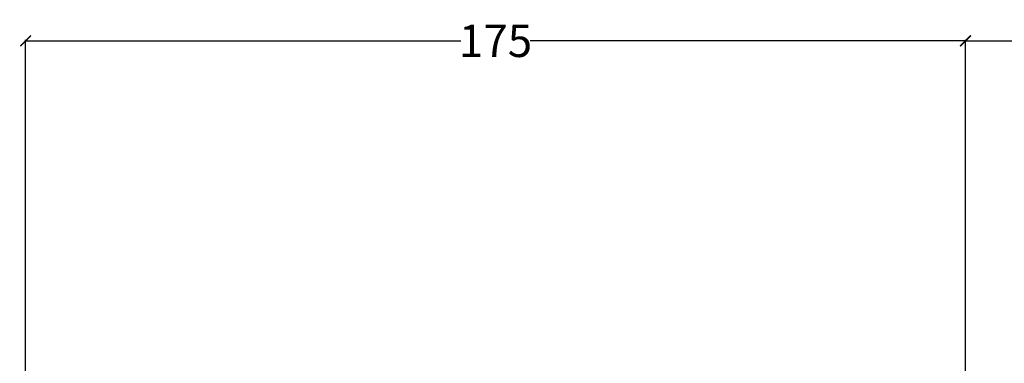
# Model space of a CAD drawing. Units: inches. Extents: x 1704 to 6393, y -157 to 1172.
# Tile 84 of 122: x 1897 to 2081, y 1045 to 1109. Entities that reach past the tile are written whole.
import ezdxf

# ---------------------------------------------------------------- set-up
doc = ezdxf.new("R2010")
doc.units = ezdxf.units.IN
doc.header["$MEASUREMENT"] = 0
doc.layers.add('A-ANNO-DIMS', color=7, linetype='Continuous', lineweight=13)
doc.styles.get("Standard").update_dxf_attribs({"font": 'arial.ttf'})
doc.dimstyles.get("Standard").update_dxf_attribs({"dimtxt": 6, "dimasz": 2, "dimexe": 0.18, "dimexo": 0.0625, "dimgap": 0.09, "dimtad": 0, "dimtih": 1, "dimtoh": 1, "dimdec": 1, "dimzin": 0, "dimdsep": 46, "dimlunit": 3, "dimtxsty": 'Standard', "dimblk": 'ARCHTICK', "dimcen": 0.09, "dimadec": 0, "dimazin": 0, "dimtfac": 1, "dimtdec": 1, "dimtofl": 0, "dimtmove": 0, "dimatfit": 3, "dimfxl": 1, "dimtolj": 1, "dimtzin": 0, "dimarcsym": 0})

# ---------------------------------------------------------------- blocks, each defined once
blk = doc.blocks.new('_ArchTick')
at = {"color": 0, "linetype": 'ByBlock', "const_width": 0.15}
blk.add_lwpolyline([(-0.5, -0.5), (0.5, 0.5)], dxfattribs=at)
blk = doc.blocks.new('*D80')
at = {"layer": 'A-ANNO-DIMS', "color": 0, "lineweight": -2, "transparency": 16777216}
for p, q in [((2018.97, 1028.92), (2016.97, 1028.92)), ((2018.97, 1025), (2018.97, 1029.1)), ((2045.49, 1028.92), (2018.97, 1028.92)), ((2045.49, 1025), (2045.49, 1029.1))]:
    blk.add_line(p, q, dxfattribs=at)
at = {"layer": 'Defpoints', "color": 0, "lineweight": -3, "transparency": 16777216}
for p in [(2018.97, 1028.92), (2018.97, 1024.94), (2045.49, 1024.94)]:
    blk.add_point(p, dxfattribs=at)
at = {"layer": 'A-ANNO-DIMS', "color": 0, "lineweight": -2, "transparency": 16777216, "xscale": 2, "yscale": 2, "zscale": 2, "rotation": 180}
blk.add_blockref('_ArchTick', (2018.97, 1028.92), dxfattribs=at)
at = {"layer": 'A-ANNO-DIMS', "color": 0, "lineweight": -2, "transparency": 16777216, "xscale": 2, "yscale": 2, "zscale": 2}
blk.add_blockref('_ArchTick', (2045.49, 1028.92), dxfattribs=at)
at = {"layer": 'A-ANNO-DIMS', "color": 0, "transparency": 16777216, "insert": (1967.17, 1028.92), "char_height": 6, "attachment_point": 5}
blk.add_mtext('\\A1;AUTUMN SHRUB 27 TYP.', dxfattribs=at)
blk = doc.blocks.new('*D92')
at = {"layer": 'A-ANNO-DIMS', "color": 0, "lineweight": -2, "transparency": 16777216}
for p, q in [((2073.35, 895.28), (2073.35, 1105.29)), ((2073.35, 1105.11), (2332.66, 1105.11)), ((2605.35, 1105.11), (2346.04, 1105.11)), ((2605.35, 895.28), (2605.35, 1105.29))]:
    blk.add_line(p, q, dxfattribs=at)
at = {"layer": 'Defpoints', "color": 0, "lineweight": -3, "transparency": 16777216}
for p in [(2605.35, 1105.11), (2073.35, 895.21), (2605.35, 895.21)]:
    blk.add_point(p, dxfattribs=at)
at = {"layer": 'A-ANNO-DIMS', "color": 0, "lineweight": -2, "transparency": 16777216, "xscale": 2, "yscale": 2, "zscale": 2, "rotation": 180}
blk.add_blockref('_ArchTick', (2073.35, 1105.11), dxfattribs=at)
at = {"layer": 'A-ANNO-DIMS', "color": 0, "lineweight": -2, "transparency": 16777216, "xscale": 2, "yscale": 2, "zscale": 2}
blk.add_blockref('_ArchTick', (2605.35, 1105.11), dxfattribs=at)
at = {"layer": 'A-ANNO-DIMS', "color": 0, "transparency": 16777216, "insert": (2339.35, 1105.11), "char_height": 6, "attachment_point": 5}
blk.add_mtext('\\A1;532', dxfattribs=at)
blk = doc.blocks.new('*D94')
at = {"layer": 'A-ANNO-DIMS', "color": 0, "lineweight": -2, "transparency": 16777216}
for p, q in [((1898.35, 895.28), (1898.35, 1105.29)), ((1898.35, 1105.11), (1979.39, 1105.11)), ((2073.35, 1105.11), (1992.31, 1105.11)), ((2073.35, 895.28), (2073.35, 1105.29))]:
    blk.add_line(p, q, dxfattribs=at)
at = {"layer": 'Defpoints', "color": 0, "lineweight": -3, "transparency": 16777216}
for p in [(2073.35, 1105.11), (1898.35, 895.21), (2073.35, 895.21)]:
    blk.add_point(p, dxfattribs=at)
at = {"layer": 'A-ANNO-DIMS', "color": 0, "lineweight": -2, "transparency": 16777216, "xscale": 2, "yscale": 2, "zscale": 2, "rotation": 180}
blk.add_blockref('_ArchTick', (1898.35, 1105.11), dxfattribs=at)
at = {"layer": 'A-ANNO-DIMS', "color": 0, "lineweight": -2, "transparency": 16777216, "xscale": 2, "yscale": 2, "zscale": 2}
blk.add_blockref('_ArchTick', (2073.35, 1105.11), dxfattribs=at)
at = {"layer": 'A-ANNO-DIMS', "color": 0, "transparency": 16777216, "insert": (1985.85, 1105.11), "char_height": 6, "attachment_point": 5}
blk.add_mtext('\\A1;175', dxfattribs=at)

msp = doc.modelspace()

# ---------------------------------------------------------------- dimensions: what is measured, and where the dimension line sits
at = {"layer": 'A-ANNO-DIMS'}
for base, p1, p2, picture, middle in [((2073.349, 1105.107), (1898.349, 895.213), (2073.349, 895.213), '*D94', (1985.849, 1105.107)), ((2605.349, 1105.107), (2073.349, 895.213), (2605.349, 895.213), '*D92', (2339.349, 1105.107))]:
    dim = msp.add_linear_dim(base=base, p1=p1, p2=p2, dimstyle='Standard', override={"dimdec": 0, "dimlfac": 1, "dimrnd": 0, "dimzin": 0, "dimdsep": 46, "dimlunit": 2}, dxfattribs=at)
    dim.commit()
    dim.dimension.update_dxf_attribs({"geometry": picture, "text_midpoint": middle})
dim = msp.add_linear_dim(base=(2018.966, 1028.916), p1=(2045.487, 1024.938), p2=(2018.966, 1024.938), angle=180, text='AUTUMN SHRUB <> TYP.', dimstyle='Standard', override={"dimdec": 0, "dimlfac": 1, "dimrnd": 0, "dimzin": 0, "dimdsep": 46, "dimlunit": 2}, dxfattribs=at)
dim.commit()
dim.dimension.update_dxf_attribs({"geometry": '*D80', "text_midpoint": (1967.173, 1028.916)})

doc.saveas('drawing.dxf')
